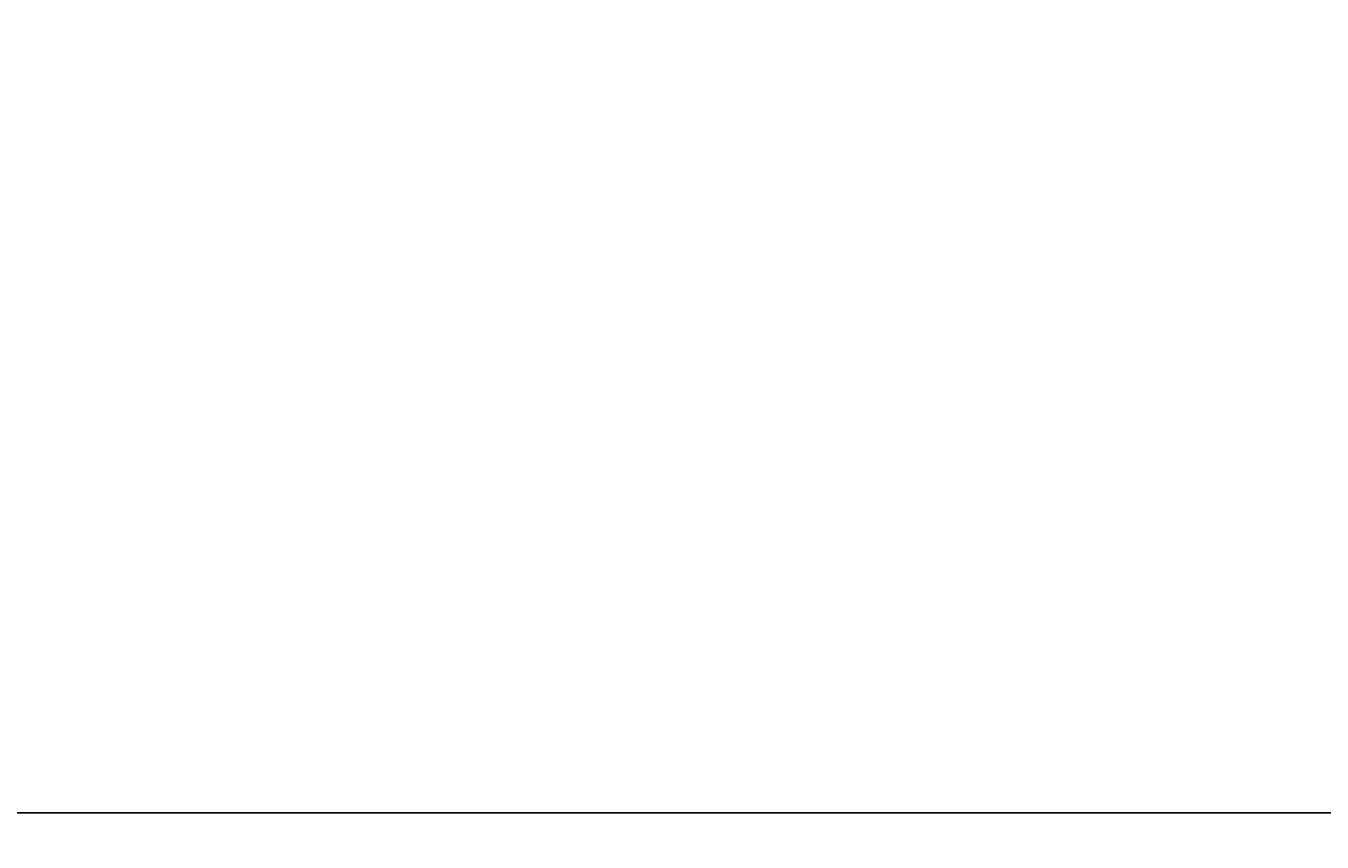
# Model space of a CAD drawing. Units: inches. Extents: x 2231 to 2461, y 2045 to 2455.
# Tile 11 of 95: x 2299 to 2326, y 2150 to 2167. Entities that reach past the tile are written whole.
import ezdxf

# ---------------------------------------------------------------- set-up
doc = ezdxf.new("R2010")
doc.units = ezdxf.units.IN
doc.layers.add('A-ANNO-DIMS', color=2, linetype='Continuous', lineweight=18)
doc.styles.get("Standard").update_dxf_attribs({"font": 'arial.ttf'})
doc.dimstyles.get("Standard").update_dxf_attribs({"dimtxt": 0.18, "dimasz": 0.18, "dimexe": 0.18, "dimexo": 0.0625, "dimgap": 0.09, "dimtad": 0, "dimtih": 1, "dimtoh": 1, "dimdec": 4, "dimzin": 0, "dimdsep": 46, "dimtxsty": 'Standard', "dimcen": 0.09, "dimadec": 0, "dimazin": 0, "dimtfac": 1, "dimtdec": 4, "dimtofl": 0, "dimtmove": 0, "dimatfit": 3, "dimfxl": 1, "dimtolj": 1, "dimtzin": 0, "dimarcsym": 0})

# ---------------------------------------------------------------- blocks, each defined once
blk = doc.blocks.new('*D51')
at = {"layer": 'A-ANNO-DIMS', "color": 0, "lineweight": -2, "transparency": 16777216}
for p, q in [((2258.794, 2306.77), (2258.794, 2044.803)), ((2330.794, 2306.77), (2330.794, 2044.803)), ((2258.974, 2044.983), (2294.576, 2044.983)), ((2330.614, 2044.983), (2295.011, 2044.983))]:
    blk.add_line(p, q, dxfattribs=at)
at = {"layer": 'A-ANNO-DIMS', "color": 0, "transparency": 16777216}
for points in [[(2258.974, 2045.013), (2258.974, 2044.953), (2258.794, 2044.983)], [(2330.614, 2045.013), (2330.614, 2044.953), (2330.794, 2044.983)]]:
    blk.add_solid(points, dxfattribs=at)
at = {"layer": 'Defpoints', "color": 0, "transparency": 16777216}
for p in [(2258.794, 2306.833), (2330.794, 2306.833), (2330.794, 2044.983)]:
    blk.add_point(p, dxfattribs=at)
at = {"layer": 'A-ANNO-DIMS', "color": 0, "transparency": 16777216, "insert": (2294.794, 2044.983), "char_height": 0.18, "attachment_point": 5}
blk.add_mtext('\\A1;72', dxfattribs=at)
blk = doc.blocks.new('*D60')
at = {"layer": 'A-ANNO-DIMS', "color": 0, "lineweight": -2, "transparency": 16777216}
for p, q in [((2432.731, 2182.833), (2230.981, 2182.833)), ((2231.161, 2182.653), (2231.161, 2166.906)), ((2231.161, 2150.795), (2231.161, 2166.542)), ((2432.731, 2150.615), (2230.981, 2150.615))]:
    blk.add_line(p, q, dxfattribs=at)
at = {"layer": 'A-ANNO-DIMS', "color": 0, "transparency": 16777216}
for points in [[(2231.131, 2182.653), (2231.191, 2182.653), (2231.161, 2182.833)], [(2231.131, 2150.795), (2231.191, 2150.795), (2231.161, 2150.615)]]:
    blk.add_solid(points, dxfattribs=at)
at = {"layer": 'Defpoints', "color": 0, "transparency": 16777216}
for p in [(2231.161, 2182.833), (2432.794, 2182.833), (2432.794, 2150.615)]:
    blk.add_point(p, dxfattribs=at)
at = {"layer": 'A-ANNO-DIMS', "color": 0, "transparency": 16777216, "insert": (2231.161, 2166.724), "char_height": 0.18, "attachment_point": 5}
blk.add_mtext('\\A1;32.22', dxfattribs=at)
blk = doc.blocks.new('*D65')
at = {"layer": 'A-ANNO-DIMS', "color": 0, "lineweight": -2, "transparency": 16777216}
for p, q in [((2285.635, 2189.285), (2285.635, 2044.803)), ((2340.667, 2189.285), (2340.667, 2044.803)), ((2285.815, 2044.983), (2312.758, 2044.983)), ((2340.487, 2044.983), (2313.545, 2044.983))]:
    blk.add_line(p, q, dxfattribs=at)
at = {"layer": 'A-ANNO-DIMS', "color": 0, "transparency": 16777216}
for points in [[(2285.815, 2045.013), (2285.815, 2044.953), (2285.635, 2044.983)], [(2340.487, 2045.013), (2340.487, 2044.953), (2340.667, 2044.983)]]:
    blk.add_solid(points, dxfattribs=at)
at = {"layer": 'Defpoints', "color": 0, "transparency": 16777216}
for p in [(2285.635, 2189.348), (2340.667, 2189.348), (2340.667, 2044.983)]:
    blk.add_point(p, dxfattribs=at)
at = {"layer": 'A-ANNO-DIMS', "color": 0, "transparency": 16777216, "insert": (2313.151, 2044.983), "char_height": 0.18, "attachment_point": 5}
blk.add_mtext('\\A1;55.03', dxfattribs=at)

msp = doc.modelspace()

# ---------------------------------------------------------------- dimensions: what is measured, and where the dimension line sits
at = {"layer": 'A-ANNO-DIMS'}
for base, p1, p2, override, picture, middle in [((2330.7935, 2044.9825), (2258.7935, 2306.8328), (2330.7935, 2306.8328), {"dimdec": 0, "dimlfac": 1, "dimrnd": 0, "dimzin": 0, "dimdsep": 46, "dimlunit": 2}, '*D51', (2294.7935, 2044.9825)), ((2340.6673, 2044.9825), (2285.6353, 2189.3477), (2340.6673, 2189.3477), {"dimdec": 2, "dimlfac": 1, "dimrnd": 0, "dimzin": 0, "dimdsep": 46, "dimlunit": 2}, '*D65', (2313.1513, 2044.9825))]:
    dim = msp.add_linear_dim(base=base, p1=p1, p2=p2, dimstyle='Standard', override=override, dxfattribs=at)
    dim.commit()
    dim.dimension.update_dxf_attribs({"geometry": picture, "text_midpoint": middle})
dim = msp.add_linear_dim(base=(2231.161, 2182.8328), p1=(2432.7935, 2150.6145), p2=(2432.7935, 2182.8328), angle=90, dimstyle='Standard', override={"dimdec": 2, "dimlfac": 1, "dimrnd": 0, "dimzin": 0, "dimdsep": 46, "dimlunit": 2}, dxfattribs=at)
dim.commit()
dim.dimension.update_dxf_attribs({"geometry": '*D60', "text_midpoint": (2231.161, 2166.7237)})

doc.saveas('drawing.dxf')
